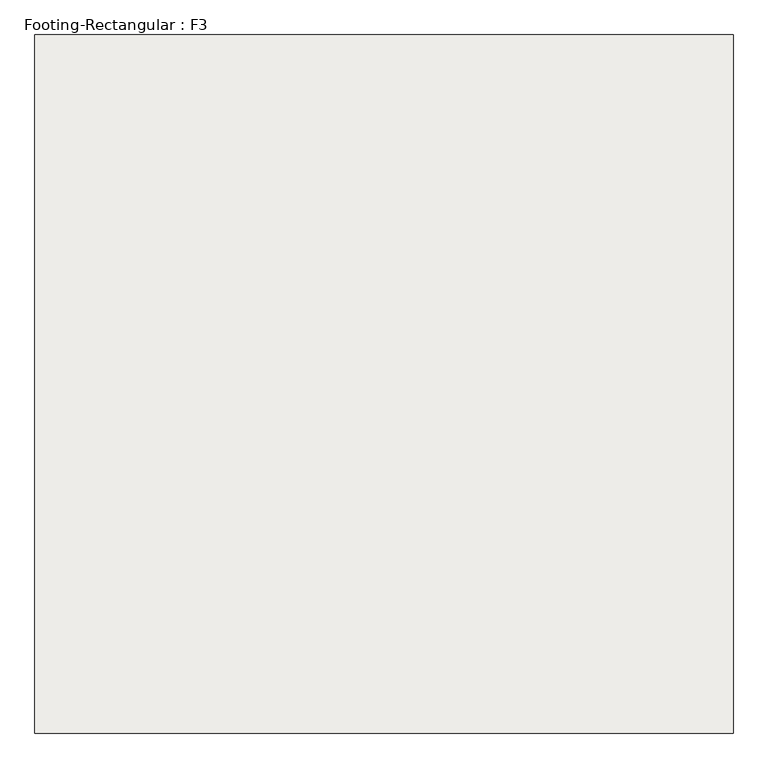
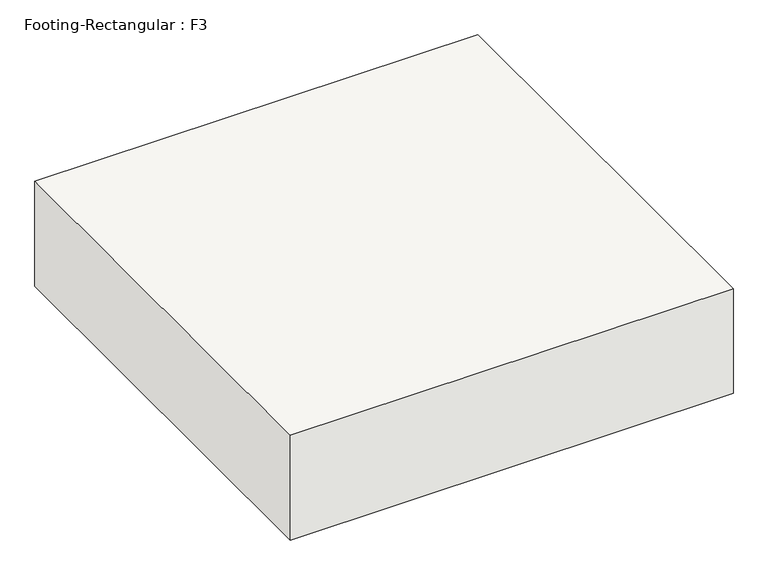
"""IFC4 building model written with IfcOpenShell, lengths in millimetres: slab geometry, Footing-Rectangular : F3."""

from ifc_helpers import new_model, si_unit, frame, origin, place, context, project, spatial, polyline, outline, extrude, source, transform, mapped, element, save


def footing_rectangular_f3_6d6a3403(model_context):
    return source(origin(), model_context, "Body", "SweptSolid", [
        extrude(outline(polyline([(914.4, 914.4), (914.4, -914.4), (-914.4, -914.4), (-914.4, 914.4), (914.4, 914.4)])), frame((0.0, 0.0, -457.2), z_axis=(0.0, 0.0, 1.0), x_axis=(1.0, 0.0, 0.0)), (0.0, 0.0, 1.0), 457.2),
    ])


if __name__ == "__main__":
    model = new_model("IFC4")
    model_context = context("Model", 3, world=origin())
    ifc_project = project(units=[si_unit("LENGTHUNIT", "METRE", prefix="MILLI")], contexts=[model_context])
    site = spatial("IfcSite", under=ifc_project)
    building = spatial("IfcBuilding", under=site)
    placement = place(None, origin())
    footing_rectangular_f3_shape = footing_rectangular_f3_6d6a3403(model_context)
    element("IfcSlab", 1, ObjectType="Footing-Rectangular : F3", at=placement, inside=building, context=model_context, shape_type="MappedRepresentation", body=[
        mapped(footing_rectangular_f3_shape, transform((0.0, 0.0, 0.0), x_axis=(1.0, 0.0, 0.0), y_axis=(0.0, 1.0, 0.0), z_axis=(0.0, 0.0, 1.0))),
    ])
    save(model, "model.ifc")

# Revit data of these elements
# Type "Footing-Rectangular : F3"
#   Width = 1828.8 mm
#   Length = 1828.8 mm
#   Foundation Thickness = 457.2 mm
#   Structural Material [instance default] = Concrete - Cast-in-Place Concrete
#   Assembly Code = ""
# Element 1 (IfcSlab, "Footing-Rectangular : F3")
#   Materials on its faces: "Concrete - Cast-in-Place Concrete"
# Materials
#   "Concrete - Cast-in-Place Concrete": class "Concrete", colour RGB 192 192 192, transparency 0, Cost = 0
